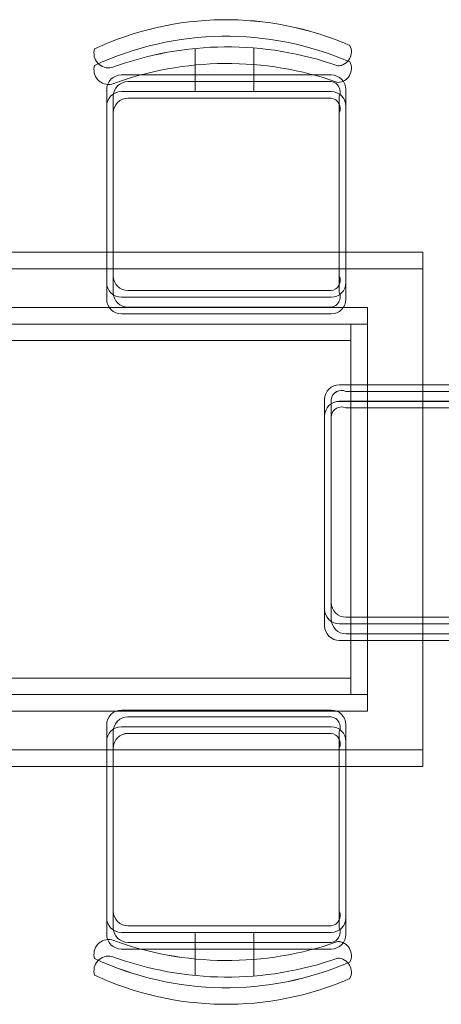
# Model space of a CAD drawing. Units: inches. Extents: x 1885 to 2748, y 783 to 2421.
# Tile 83 of 117: x 2156 to 2176, y 2066 to 2111. Entities that reach past the tile are written whole.
import ezdxf

# ---------------------------------------------------------------- set-up
doc = ezdxf.new("R2010")
doc.units = ezdxf.units.IN
doc.layers.add('A-FURN', color=8, linetype='Continuous', lineweight=13)

# ---------------------------------------------------------------- blocks, each defined once
blk = doc.blocks.new('TABLE-DINING-RECT')
for points in [[(-0.004, 23.421), (37.776, 23.421), (37.776, 0.754), (-0.004, 0.754)], [(-0.004, 23.421), (37.776, 23.421), (37.776, 0.753), (-0.004, 0.753)], [(-0.004, 22.666), (37.776, 22.666), (37.776, -0.002), (-0.004, -0.002)], [(-0.004, 22.665), (37.776, 22.665), (37.776, -0.002), (-0.004, -0.002)], [(2.515, 20.903), (35.257, 20.903), (35.257, 3.272), (2.515, 3.272)], [(2.515, 20.902), (35.257, 20.902), (35.257, 3.272), (2.515, 3.272)], [(2.515, 20.147), (35.257, 20.147), (35.257, 2.517), (2.515, 2.517)], [(2.515, 20.147), (35.257, 20.147), (35.257, 2.516), (2.515, 2.516)], [(3.27, 20.147), (34.501, 20.147), (34.501, 4.028), (3.27, 4.028)], [(3.27, 20.147), (34.501, 20.147), (34.501, 4.027), (3.27, 4.027)], [(3.27, 19.391), (34.501, 19.391), (34.501, 3.272), (3.27, 3.272)], [(3.27, 19.391), (34.501, 19.391), (34.501, 3.272), (3.27, 3.272)]]:
    blk.add_lwpolyline(points, close=True)
blk = doc.blocks.new('CHAIR-DINING-END')
for points in [[(10.121, 11.561, 0.414214), (9.453, 12.229), (0.669, 12.229, 0.414214), (0.001, 11.561), (0.001, 2.008, 0.414214), (0.669, 1.34), (9.453, 1.34, 0.414214), (10.121, 2.008), (10.121, 11.561)], [(10.121, 11.56, 0.414214), (9.453, 12.229), (0.669, 12.229, 0.414214), (0.001, 11.56), (0.001, 2.007, 0.414214), (0.669, 1.339), (9.453, 1.339, 0.414214), (10.121, 2.007), (10.121, 11.56)], [(10.534, 11.861, -0.175809), (10.456, 1.571, 0.578392), (11.313, 0.792, 0.214524), (11.469, 12.407, 0.552014), (10.534, 11.861, -0.065079)], [(10.534, 11.861, -0.175809), (10.456, 1.571, 0.578392), (11.313, 0.791, 0.214524), (11.469, 12.407, 0.552014), (10.534, 11.861, -0.065079)], [(10.534, 11.106, -0.175809), (10.456, 0.816, 0.578392), (11.313, 0.036, 0.214524), (11.469, 11.651, 0.552014), (10.534, 11.106, -0.065079)], [(10.534, 11.105, -0.175809), (10.456, 0.815, 0.578392), (11.313, 0.036, 0.214524), (11.469, 11.651, 0.552014), (10.534, 11.105, -0.065079)], [(10.121, 10.805, 0.414214), (9.453, 11.474), (0.669, 11.474, 0.414214), (0.001, 10.805), (0.001, 1.252, 0.414214), (0.669, 0.584), (9.453, 0.584, 0.414214), (10.121, 1.252), (10.121, 10.805)], [(10.121, 10.805, 0.414214), (9.453, 11.473), (0.669, 11.473, 0.414214), (0.001, 10.805), (0.001, 1.252, 0.414214), (0.669, 0.584), (9.453, 0.584, 0.414214), (10.121, 1.252), (10.121, 10.805)], [(10.121, 5.363), (11.329, 5.363, -0.064759)], [(10.121, 5.363), (11.329, 5.363, -0.064759)], [(10.121, 4.608), (11.329, 4.608, -0.064759)], [(10.121, 4.607), (11.329, 4.607, -0.064759)]]:
    blk.add_lwpolyline(points, format="xyb")
for points in [[(9.82, 11.557), (9.82, 2.309, -0.414214), (9.152, 1.641), (0.97, 1.641, -0.414214), (0.302, 2.309), (0.302, 11.557, -0.512069), (0.97, 11.928), (9.152, 11.928, -0.512069)], [(9.82, 11.556), (9.82, 2.309, -0.414214), (9.152, 1.64), (0.97, 1.64, -0.414214), (0.302, 2.309), (0.302, 11.556, -0.512069), (0.97, 11.928), (9.152, 11.928, -0.512069)], [(9.82, 10.801), (9.82, 1.553, -0.414214), (9.152, 0.885), (0.97, 0.885, -0.414214), (0.302, 1.553), (0.302, 10.801, -0.512069), (0.97, 11.172), (9.152, 11.172, -0.512069)], [(9.82, 10.801), (9.82, 1.553, -0.414214), (9.152, 0.885), (0.97, 0.885, -0.414214), (0.302, 1.553), (0.302, 10.801, -0.512069), (0.97, 11.172), (9.152, 11.172, -0.512069)]]:
    blk.add_lwpolyline(points, format="xyb", close=True)
for points in [[(11.351, 8.037), (10.121, 8.037)], [(11.351, 8.037), (10.121, 8.037)], [(11.351, 7.282), (10.121, 7.282)], [(11.351, 7.281), (10.121, 7.281)]]:
    blk.add_lwpolyline(points)

msp = doc.modelspace()

# ---------------------------------------------------------------- linework, layer by layer
at = {"layer": 'A-FURN'}
for points in [[(2160.636, 2109.014, -0.578392), (2159.856, 2109.871, -0.214524), (2171.472, 2110.027, -0.552014), (2170.926, 2109.092, 0.175809), (2160.636, 2109.014)], [(2160.636, 2109.013, -0.578392), (2159.856, 2109.87, -0.214524), (2171.472, 2110.026, -0.552014), (2170.926, 2109.091, 0.175809), (2160.636, 2109.013)], [(2160.636, 2108.258, -0.578392), (2159.856, 2109.115, -0.214524), (2171.472, 2109.271, -0.552014), (2170.926, 2108.336, 0.175809), (2160.636, 2108.258)], [(2160.636, 2108.258, -0.578392), (2159.856, 2109.115, -0.214524), (2171.472, 2109.271, -0.552014), (2170.926, 2108.336, 0.175809), (2160.636, 2108.258)], [(2164.428, 2108.679), (2164.428, 2109.887, 0.064759)], [(2164.428, 2108.678), (2164.428, 2109.886, 0.064759)], [(2164.428, 2107.923), (2164.428, 2109.131, 0.064759)], [(2164.428, 2107.923), (2164.428, 2109.131, 0.064759)], [(2170.625, 2108.679, -0.414214), (2171.294, 2108.01), (2171.294, 2099.227, -0.414214), (2170.625, 2098.558), (2161.072, 2098.558, -0.414214), (2160.404, 2099.227), (2160.404, 2108.01, -0.414214), (2161.072, 2108.679), (2170.625, 2108.679)], [(2170.625, 2108.678, -0.414214), (2171.294, 2108.01), (2171.294, 2099.226, -0.414214), (2170.625, 2098.558), (2161.072, 2098.558, -0.414214), (2160.404, 2099.226), (2160.404, 2108.01, -0.414214), (2161.072, 2108.678), (2170.625, 2108.678)], [(2170.625, 2107.923, -0.414214), (2171.294, 2107.255), (2171.294, 2098.471, -0.414214), (2170.625, 2097.803), (2161.072, 2097.803, -0.414214), (2160.404, 2098.471), (2160.404, 2107.255, -0.414214), (2161.072, 2107.923), (2170.625, 2107.923)], [(2170.625, 2107.923, -0.414214), (2171.294, 2107.254), (2171.294, 2098.471, -0.414214), (2170.625, 2097.802), (2161.072, 2097.802, -0.414214), (2160.404, 2098.471), (2160.404, 2107.254, -0.414214), (2161.072, 2107.923), (2170.625, 2107.923)], [(2170.625, 2069.633, 0.414214), (2171.294, 2070.301), (2171.294, 2079.085, 0.414214), (2170.625, 2079.753), (2161.072, 2079.753, 0.414214), (2160.404, 2079.085), (2160.404, 2070.301, 0.414214), (2161.072, 2069.633), (2170.625, 2069.633)], [(2170.625, 2069.632, 0.414214), (2171.294, 2070.301), (2171.294, 2079.085, 0.414214), (2170.625, 2079.753), (2161.072, 2079.753, 0.414214), (2160.404, 2079.085), (2160.404, 2070.301, 0.414214), (2161.072, 2069.632), (2170.625, 2069.632)], [(2170.625, 2068.877, 0.414214), (2171.294, 2069.546), (2171.294, 2078.329, 0.414214), (2170.625, 2078.998), (2161.072, 2078.998, 0.414214), (2160.404, 2078.329), (2160.404, 2069.546, 0.414214), (2161.072, 2068.877), (2170.625, 2068.877)], [(2170.625, 2068.877, 0.414214), (2171.294, 2069.545), (2171.294, 2078.329, 0.414214), (2170.625, 2078.997), (2161.072, 2078.997, 0.414214), (2160.404, 2078.329), (2160.404, 2069.545, 0.414214), (2161.072, 2068.877), (2170.625, 2068.877)], [(2170.926, 2069.22, -0.175809), (2160.636, 2069.298, 0.578392), (2159.856, 2068.441, 0.214524), (2171.472, 2068.285, 0.552014), (2170.926, 2069.22, -0.065079)], [(2170.926, 2069.219, -0.175809), (2160.636, 2069.297, 0.578392), (2159.856, 2068.44, 0.214524), (2171.472, 2068.284, 0.552014), (2170.926, 2069.219, -0.065079)], [(2164.428, 2069.633), (2164.428, 2068.425, -0.064759)], [(2164.428, 2069.632), (2164.428, 2068.424, -0.064759)], [(2164.428, 2068.877), (2164.428, 2067.669, -0.064759)], [(2164.428, 2068.877), (2164.428, 2067.669, -0.064759)], [(2170.926, 2068.464, -0.175809), (2160.636, 2068.542, 0.578392), (2159.856, 2067.685, 0.214524), (2171.472, 2067.529, 0.552014), (2170.926, 2068.464, -0.065079)], [(2170.926, 2068.464, -0.175809), (2160.636, 2068.542, 0.578392), (2159.856, 2067.685, 0.214524), (2171.472, 2067.529, 0.552014), (2170.926, 2068.464, -0.065079)]]:
    msp.add_lwpolyline(points, format="xyb", dxfattribs=at)
for points in [[(2167.102, 2109.909), (2167.102, 2108.679)], [(2167.102, 2109.908), (2167.102, 2108.678)], [(2167.102, 2109.153), (2167.102, 2107.923)], [(2167.102, 2109.153), (2167.102, 2107.923)], [(2167.102, 2068.403), (2167.102, 2069.633)], [(2167.102, 2068.402), (2167.102, 2069.632)], [(2167.102, 2067.647), (2167.102, 2068.877)], [(2167.102, 2067.647), (2167.102, 2068.877)]]:
    msp.add_lwpolyline(points, dxfattribs=at)
for points in [[(2170.621, 2108.378), (2161.374, 2108.378, 0.414214), (2160.705, 2107.709), (2160.705, 2099.528, 0.414214), (2161.374, 2098.859), (2170.621, 2098.859, 0.512069), (2170.993, 2099.528), (2170.993, 2107.709, 0.512069)], [(2170.621, 2108.377), (2161.374, 2108.377, 0.414214), (2160.705, 2107.709), (2160.705, 2099.527, 0.414214), (2161.374, 2098.859), (2170.621, 2098.859, 0.512069), (2170.993, 2099.527), (2170.993, 2107.709, 0.512069)], [(2170.621, 2107.622), (2161.374, 2107.622, 0.414214), (2160.705, 2106.954), (2160.705, 2098.772, 0.414214), (2161.374, 2098.104), (2170.621, 2098.104, 0.512069), (2170.993, 2098.772), (2170.993, 2106.954, 0.512069)], [(2170.621, 2107.622), (2161.374, 2107.622, 0.414214), (2160.705, 2106.953), (2160.705, 2098.772, 0.414214), (2161.374, 2098.103), (2170.621, 2098.103, 0.512069), (2170.993, 2098.772), (2170.993, 2106.953, 0.512069)], [(2170.621, 2069.934), (2161.374, 2069.934, -0.414214), (2160.705, 2070.602), (2160.705, 2078.784, -0.414214), (2161.374, 2079.452), (2170.621, 2079.452, -0.512069), (2170.993, 2078.784), (2170.993, 2070.602, -0.512069)], [(2170.621, 2069.934), (2161.374, 2069.934, -0.414214), (2160.705, 2070.602), (2160.705, 2078.783, -0.414214), (2161.374, 2079.452), (2170.621, 2079.452, -0.512069), (2170.993, 2078.783), (2170.993, 2070.602, -0.512069)], [(2170.621, 2069.178), (2161.374, 2069.178, -0.414214), (2160.705, 2069.847), (2160.705, 2078.028, -0.414214), (2161.374, 2078.697), (2170.621, 2078.697, -0.512069), (2170.993, 2078.028), (2170.993, 2069.847, -0.512069)], [(2170.621, 2069.178), (2161.374, 2069.178, -0.414214), (2160.705, 2069.846), (2160.705, 2078.028, -0.414214), (2161.374, 2078.696), (2170.621, 2078.696, -0.512069), (2170.993, 2078.028), (2170.993, 2069.846, -0.512069)]]:
    msp.add_lwpolyline(points, format="xyb", close=True, dxfattribs=at)

# ---------------------------------------------------------------- block references
for name, p in [('TABLE-DINING-RECT', (2137.014, 2077.19)), ('CHAIR-DINING-END', (2170.325, 2082.344))]:
    msp.add_blockref(name, p, dxfattribs=at)

doc.saveas('drawing.dxf')
